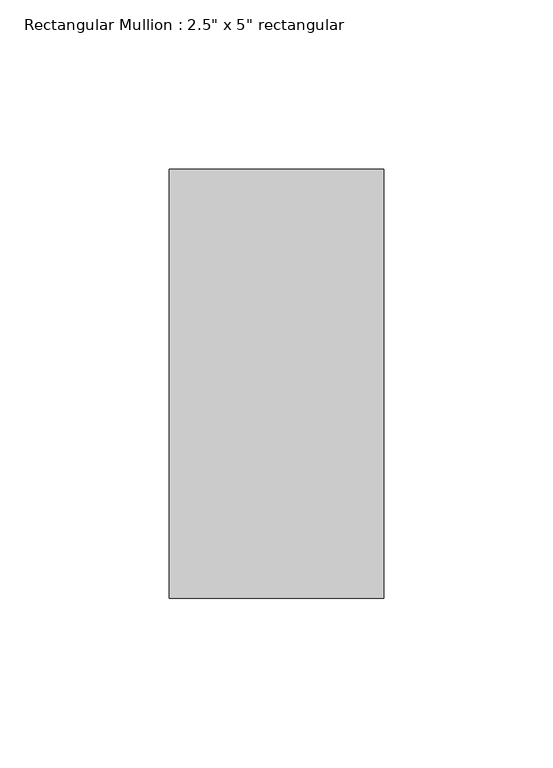
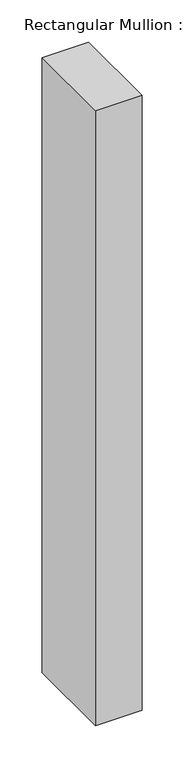
"""IFC4 building model written with IfcOpenShell, lengths in millimetres: member geometry."""

from ifc_helpers import new_model, si_unit, frame, origin, place, context, project, spatial, polyline, outline, extrude, source, transform, mapped, element, save


def member_d6486fbc(model_context):
    return source(origin(), model_context, "Body", "SweptSolid", [
        extrude(outline(polyline([(31.75, 63.5), (31.75, -63.5), (-31.75, -63.5), (-31.75, 63.5), (31.75, 63.5)])), frame((0.0, 0.0, -889.6989237), z_axis=(0.0, 0.0, 1.0), x_axis=(1.0, 0.0, 0.0)), (0.0, 0.0, 1.0), 889.6989237),
    ])


if __name__ == "__main__":
    model = new_model("IFC4")
    model_context = context("Model", 3, world=origin())
    ifc_project = project(units=[si_unit("LENGTHUNIT", "METRE", prefix="MILLI")], contexts=[model_context])
    site = spatial("IfcSite", under=ifc_project)
    building = spatial("IfcBuilding", under=site)
    placement = place(None, origin())
    member_shape = member_d6486fbc(model_context)
    element("IfcMember", 1, ObjectType="Rectangular Mullion : 2.5\" x 5\" rectangular", at=placement, inside=building, context=model_context, shape_type="MappedRepresentation", body=[
        mapped(member_shape, transform((0.0, 0.0, 0.0), x_axis=(1.0, 0.0, 0.0), y_axis=(0.0, 1.0, 0.0), z_axis=(0.0, 0.0, 1.0))),
    ])
    save(model, "model.ifc")

# Revit data of these elements
# Type "Rectangular Mullion : 2.5\" x 5\" rectangular"
#   built-in parameter 1007304 = 0.416667 (stored number, unit not read)
#   built-in parameter 1007301 = 0.104167 (stored number, unit not read)
#   built-in parameter 1007300 = 0.104167 (stored number, unit not read)
# Element 1 (IfcMember, "Rectangular Mullion : 2.5\" x 5\" rectangular")
#   Materials on its faces: "Aluminum"
# Materials
#   "Aluminum": class "Metal", colour RGB 247 247 247, transparency 0, Description = "Aluminum 6061", Cost = 0
